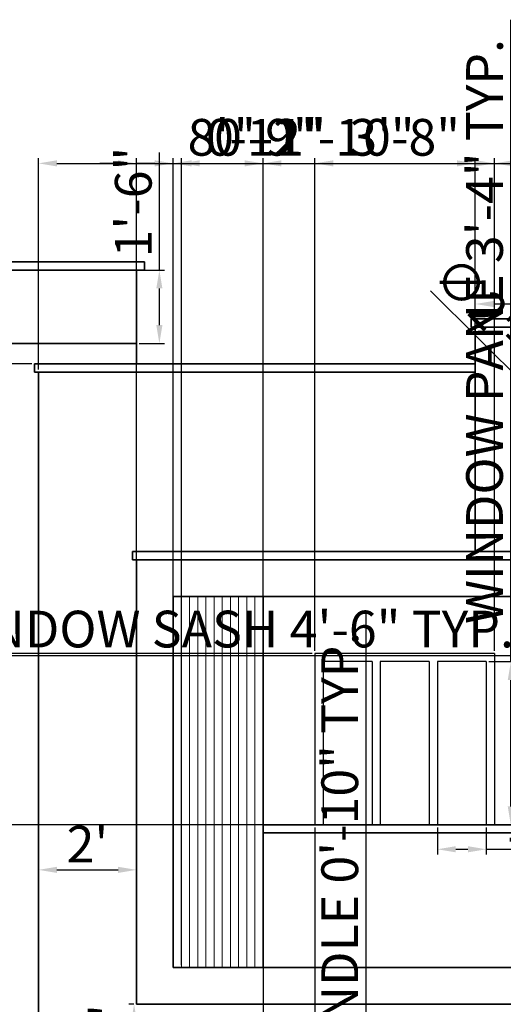
# Model space of a CAD drawing. Units: inches. Extents: x 3297 to 3846, y 520 to 959.
# Tile 4 of 5: x 3483 to 3602, y 717 to 959. Entities that reach past the tile are written whole.
import ezdxf

# ---------------------------------------------------------------- set-up
doc = ezdxf.new("R2010")
doc.units = ezdxf.units.IN
for name, color, linetype, lineweight in [('A-ANNO-DIMS', 2, 'Continuous', 18), ('A-ELEV', 7, 'Continuous', 35), ('A-ELEV-PATT', 8, 'Continuous', 13), ('A-GLAZ', 3, 'Continuous', 25)]:
    doc.layers.add(name, color=color, linetype=linetype, lineweight=lineweight)
doc.styles.get("Standard").update_dxf_attribs({"font": 'arial.ttf'})
doc.dimstyles.new('ISO-25', dxfattribs={"dimtxt": 9, "dimasz": 4.5, "dimexe": 1.25, "dimexo": 0.625, "dimtad": 1, "dimdec": 0, "dimlunit": 3, "dimtxsty": 'Standard', "dimcen": 2.5, "dimadec": 0, "dimazin": 0, "dimtfac": 1, "dimtdec": 0, "dimtmove": 0, "dimatfit": 3, "dimfxl": 1, "dimarcsym": 0})

# ---------------------------------------------------------------- blocks, each defined once
blk = doc.blocks.new('*D4')
at = {"layer": 'A-ANNO-DIMS', "color": 0, "lineweight": -2, "transparency": 16777216}
for p, q in [((3517.67, 897.24), (3517.67, 926.07)), ((3512.69, 897.24), (3518.92, 897.24)), ((3517.67, 883.74), (3517.67, 892.74)), ((3512.69, 879.24), (3518.92, 879.24))]:
    blk.add_line(p, q, dxfattribs=at)
at = {"layer": 'A-ANNO-DIMS', "color": 0, "transparency": 16777216}
for points in [[(3516.92, 892.74), (3518.42, 892.74), (3517.67, 897.24)], [(3516.92, 883.74), (3518.42, 883.74), (3517.67, 879.24)]]:
    blk.add_solid(points, dxfattribs=at)
at = {"layer": 'Defpoints', "color": 0, "transparency": 16777216}
for p in [(3512.06, 897.24), (3517.67, 897.24), (3512.06, 879.24)]:
    blk.add_point(p, dxfattribs=at)
at = {"layer": 'A-ANNO-DIMS', "color": 0, "transparency": 16777216, "insert": (3512.45, 913.9), "char_height": 9, "attachment_point": 5, "rotation": 90}
blk.add_mtext('1\'-6"', dxfattribs=at)
blk = doc.blocks.new('*D16')
at = {"layer": 'A-ANNO-DIMS', "color": 0, "lineweight": -2, "transparency": 16777216}
for p, q in [((3595.06, 874.87), (3595.06, 890.17)), ((3599.56, 888.92), (3650.56, 888.92)), ((3655.06, 874.87), (3655.06, 890.17))]:
    blk.add_line(p, q, dxfattribs=at)
at = {"layer": 'A-ANNO-DIMS', "color": 0, "transparency": 16777216}
for points in [[(3599.56, 889.67), (3599.56, 888.17), (3595.06, 888.92)], [(3650.56, 889.67), (3650.56, 888.17), (3655.06, 888.92)]]:
    blk.add_solid(points, dxfattribs=at)
at = {"layer": 'Defpoints', "color": 0, "transparency": 16777216}
for p in [(3655.06, 888.92), (3595.06, 874.24), (3655.06, 874.24)]:
    blk.add_point(p, dxfattribs=at)
at = {"layer": 'A-ANNO-DIMS', "color": 0, "transparency": 16777216, "insert": (3625.06, 894.12), "char_height": 9, "attachment_point": 5}
blk.add_mtext("5'", dxfattribs=at)
blk = doc.blocks.new('*D18')
at = {"layer": 'A-ANNO-DIMS', "color": 0, "lineweight": -2, "transparency": 16777216}
for p, q in [((3488.06, 746.43), (3488.06, 751.45)), ((3512.06, 746.43), (3512.06, 751.45)), ((3492.56, 750.2), (3507.56, 750.2))]:
    blk.add_line(p, q, dxfattribs=at)
at = {"layer": 'A-ANNO-DIMS', "color": 0, "transparency": 16777216}
for points in [[(3492.56, 750.95), (3492.56, 749.45), (3488.06, 750.2)], [(3507.56, 750.95), (3507.56, 749.45), (3512.06, 750.2)]]:
    blk.add_solid(points, dxfattribs=at)
at = {"layer": 'Defpoints', "color": 0, "transparency": 16777216}
for p in [(3512.06, 750.2), (3488.06, 745.81), (3512.06, 745.81)]:
    blk.add_point(p, dxfattribs=at)
at = {"layer": 'A-ANNO-DIMS', "color": 0, "transparency": 16777216, "insert": (3500.06, 755.34), "char_height": 9, "attachment_point": 5}
blk.add_mtext("2'", dxfattribs=at)
blk = doc.blocks.new('*D19')
at = {"layer": 'A-ANNO-DIMS', "color": 0, "lineweight": -2, "transparency": 16777216}
for p, q in [((3511.44, 717.24), (3510.23, 717.24)), ((3511.48, 712.74), (3511.48, 694.74)), ((3511.44, 690.24), (3510.23, 690.24))]:
    blk.add_line(p, q, dxfattribs=at)
at = {"layer": 'A-ANNO-DIMS', "color": 0, "transparency": 16777216}
for points in [[(3510.73, 712.74), (3512.23, 712.74), (3511.48, 717.24)], [(3510.73, 694.74), (3512.23, 694.74), (3511.48, 690.24)]]:
    blk.add_solid(points, dxfattribs=at)
at = {"layer": 'Defpoints', "color": 0, "transparency": 16777216}
for p in [(3512.06, 717.24), (3511.48, 690.24), (3512.06, 690.24)]:
    blk.add_point(p, dxfattribs=at)
at = {"layer": 'A-ANNO-DIMS', "color": 0, "transparency": 16777216, "insert": (3506.25, 703.74), "char_height": 9, "attachment_point": 5, "rotation": 90}
blk.add_mtext('2\'-3"', dxfattribs=at)
blk = doc.blocks.new('WIN-PANE')
for p, q in [((12, 40), (0, 40)), ((0, 40), (0, 0)), ((12, 40), (12, 0))]:
    blk.add_line(p, q)
blk = doc.blocks.new('*D27')
at = {"layer": 'A-ANNO-DIMS', "color": 0, "lineweight": -2, "transparency": 16777216}
for p, q in [((3603.76, 801.24), (3603.76, 958.61)), ((3598.39, 801.24), (3605.01, 801.24)), ((3603.76, 765.74), (3603.76, 796.74)), ((3598.39, 761.24), (3605.01, 761.24))]:
    blk.add_line(p, q, dxfattribs=at)
at = {"layer": 'A-ANNO-DIMS', "color": 0, "transparency": 16777216}
for points in [[(3603.01, 796.74), (3604.51, 796.74), (3603.76, 801.24)], [(3603.01, 765.74), (3604.51, 765.74), (3603.76, 761.24)]]:
    blk.add_solid(points, dxfattribs=at)
at = {"layer": 'Defpoints', "color": 0, "transparency": 16777216}
for p in [(3597.76, 801.24), (3603.76, 801.24), (3597.76, 761.24)]:
    blk.add_point(p, dxfattribs=at)
at = {"layer": 'A-ANNO-DIMS', "color": 0, "transparency": 16777216, "insert": (3598.48, 882.18), "char_height": 9, "attachment_point": 5, "rotation": 90}
blk.add_mtext('WINDOW PANE 3\'-4" TYP.', dxfattribs=at)
blk = doc.blocks.new('*D28')
at = {"layer": 'A-ANNO-DIMS', "color": 0, "lineweight": -2, "transparency": 16777216}
for p, q in [((3585.76, 760.62), (3585.76, 753.99)), ((3597.76, 760.62), (3597.76, 753.99)), ((3590.26, 755.24), (3593.26, 755.24)), ((3597.76, 755.24), (3657.53, 755.24))]:
    blk.add_line(p, q, dxfattribs=at)
at = {"layer": 'A-ANNO-DIMS', "color": 0, "transparency": 16777216}
for points in [[(3590.26, 755.99), (3590.26, 754.49), (3585.76, 755.24)], [(3593.26, 755.99), (3593.26, 754.49), (3597.76, 755.24)]]:
    blk.add_solid(points, dxfattribs=at)
at = {"layer": 'Defpoints', "color": 0, "transparency": 16777216}
for p in [(3585.76, 761.24), (3597.76, 761.24), (3597.76, 755.24)]:
    blk.add_point(p, dxfattribs=at)
at = {"layer": 'A-ANNO-DIMS', "color": 0, "transparency": 16777216, "insert": (3629.89, 760.46), "char_height": 9, "attachment_point": 5}
blk.add_mtext('1\'-0" TYP.', dxfattribs=at)
blk = doc.blocks.new('*D29')
at = {"layer": 'A-ANNO-DIMS', "color": 0, "lineweight": -2, "transparency": 16777216}
for p, q in [((3568.3, 650.24), (3568.3, 813.1)), ((3569.18, 645.74), (3567.05, 645.74)), ((3568.3, 635.74), (3568.3, 645.74)), ((3569.18, 635.74), (3567.05, 635.74)), ((3568.3, 631.24), (3568.3, 626.74))]:
    blk.add_line(p, q, dxfattribs=at)
at = {"layer": 'A-ANNO-DIMS', "color": 0, "transparency": 16777216}
for points in [[(3567.55, 650.24), (3569.05, 650.24), (3568.3, 645.74)], [(3567.55, 631.24), (3569.05, 631.24), (3568.3, 635.74)]]:
    blk.add_solid(points, dxfattribs=at)
at = {"layer": 'Defpoints', "color": 0, "transparency": 16777216}
for p in [(3568.3, 645.74), (3569.8, 645.74), (3569.8, 635.74)]:
    blk.add_point(p, dxfattribs=at)
at = {"layer": 'A-ANNO-DIMS', "color": 0, "transparency": 16777216, "insert": (3563.02, 733.92), "char_height": 9, "attachment_point": 5, "rotation": 90}
blk.add_mtext('DOOR HANDLE 0\'-10" TYP.', dxfattribs=at)
blk = doc.blocks.new('*D33')
at = {"layer": 'A-ANNO-DIMS', "color": 0, "lineweight": -2, "transparency": 16777216}
for p, q in [((3398.06, 795.31), (3398.06, 804.03)), ((3452.06, 795.31), (3452.06, 804.03)), ((3402.56, 802.78), (3447.56, 802.78)), ((3452.06, 802.78), (3609.43, 802.78))]:
    blk.add_line(p, q, dxfattribs=at)
at = {"layer": 'A-ANNO-DIMS', "color": 0, "transparency": 16777216}
for points in [[(3402.56, 803.53), (3402.56, 802.03), (3398.06, 802.78)], [(3447.56, 803.53), (3447.56, 802.03), (3452.06, 802.78)]]:
    blk.add_solid(points, dxfattribs=at)
at = {"layer": 'Defpoints', "color": 0, "transparency": 16777216}
for p in [(3452.06, 802.78), (3398.06, 794.68), (3452.06, 794.68)]:
    blk.add_point(p, dxfattribs=at)
at = {"layer": 'A-ANNO-DIMS', "color": 0, "transparency": 16777216, "insert": (3533, 808.06), "char_height": 9, "attachment_point": 5}
blk.add_mtext('WINDOW SASH 4\'-6" TYP.', dxfattribs=at)
blk = doc.blocks.new('*D43')
at = {"layer": 'A-ANNO-DIMS', "color": 0, "lineweight": -2, "transparency": 16777216}
for p, q in [((3488.06, 872.87), (3488.06, 924.64)), ((3595.06, 883.87), (3595.06, 924.64)), ((3492.56, 923.39), (3590.56, 923.39))]:
    blk.add_line(p, q, dxfattribs=at)
at = {"layer": 'A-ANNO-DIMS', "color": 0, "transparency": 16777216}
for points in [[(3492.56, 924.14), (3492.56, 922.64), (3488.06, 923.39)], [(3590.56, 924.14), (3590.56, 922.64), (3595.06, 923.39)]]:
    blk.add_solid(points, dxfattribs=at)
at = {"layer": 'Defpoints', "color": 0, "transparency": 16777216}
for p in [(3595.06, 923.39), (3595.06, 883.24), (3488.06, 872.24)]:
    blk.add_point(p, dxfattribs=at)
at = {"layer": 'A-ANNO-DIMS', "color": 0, "transparency": 16777216, "insert": (3541.56, 928.61), "char_height": 9, "attachment_point": 5}
blk.add_mtext('8\'-11"', dxfattribs=at)
blk = doc.blocks.new('*D64')
at = {"layer": 'A-ANNO-DIMS', "color": 0, "lineweight": -2, "transparency": 16777216}
for p, q in [((3512.06, 732.87), (3512.06, 924.64)), ((3521.06, 726.87), (3521.06, 924.64)), ((3507.56, 923.39), (3503.06, 923.39)), ((3512.06, 923.39), (3521.06, 923.39)), ((3525.56, 923.39), (3555.24, 923.39))]:
    blk.add_line(p, q, dxfattribs=at)
at = {"layer": 'A-ANNO-DIMS', "color": 0, "transparency": 16777216}
for points in [[(3507.56, 924.14), (3507.56, 922.64), (3512.06, 923.39)], [(3525.56, 924.14), (3525.56, 922.64), (3521.06, 923.39)]]:
    blk.add_solid(points, dxfattribs=at)
at = {"layer": 'Defpoints', "color": 0, "transparency": 16777216}
for p in [(3521.06, 923.39), (3512.06, 732.24), (3521.06, 726.24)]:
    blk.add_point(p, dxfattribs=at)
at = {"layer": 'A-ANNO-DIMS', "color": 0, "transparency": 16777216, "insert": (3542.65, 928.61), "char_height": 9, "attachment_point": 5}
blk.add_mtext('0\'-9"', dxfattribs=at)
blk = doc.blocks.new('*D65')
at = {"layer": 'A-ANNO-DIMS', "color": 0, "lineweight": -2, "transparency": 16777216}
for p, q in [((3521.06, 817.87), (3521.06, 924.64)), ((3543.06, 817.87), (3543.06, 924.64)), ((3525.56, 923.39), (3538.56, 923.39)), ((3543.06, 923.39), (3578.88, 923.39))]:
    blk.add_line(p, q, dxfattribs=at)
at = {"layer": 'A-ANNO-DIMS', "color": 0, "transparency": 16777216}
for points in [[(3525.56, 924.14), (3525.56, 922.64), (3521.06, 923.39)], [(3538.56, 924.14), (3538.56, 922.64), (3543.06, 923.39)]]:
    blk.add_solid(points, dxfattribs=at)
at = {"layer": 'Defpoints', "color": 0, "transparency": 16777216}
for p in [(3543.06, 923.39), (3521.06, 817.24), (3543.06, 817.24)]:
    blk.add_point(p, dxfattribs=at)
at = {"layer": 'A-ANNO-DIMS', "color": 0, "transparency": 16777216, "insert": (3563.22, 928.61), "char_height": 9, "attachment_point": 5}
blk.add_mtext('1\'-10"', dxfattribs=at)
blk = doc.blocks.new('*D66')
at = {"layer": 'A-ANNO-DIMS', "color": 0, "lineweight": -2, "transparency": 16777216}
for p, q in [((3521.06, 726.87), (3521.06, 924.64)), ((3523.06, 726.87), (3523.06, 924.64)), ((3516.56, 923.39), (3512.06, 923.39)), ((3521.06, 923.39), (3523.06, 923.39)), ((3527.56, 923.39), (3557.24, 923.39))]:
    blk.add_line(p, q, dxfattribs=at)
at = {"layer": 'A-ANNO-DIMS', "color": 0, "transparency": 16777216}
for points in [[(3516.56, 924.14), (3516.56, 922.64), (3521.06, 923.39)], [(3527.56, 924.14), (3527.56, 922.64), (3523.06, 923.39)]]:
    blk.add_solid(points, dxfattribs=at)
at = {"layer": 'Defpoints', "color": 0, "transparency": 16777216}
for p in [(3523.06, 923.39), (3521.06, 726.24), (3523.06, 726.24)]:
    blk.add_point(p, dxfattribs=at)
at = {"layer": 'A-ANNO-DIMS', "color": 0, "transparency": 16777216, "insert": (3544.65, 928.61), "char_height": 9, "attachment_point": 5}
blk.add_mtext('0\'-2"', dxfattribs=at)
blk = doc.blocks.new('*D69')
at = {"layer": 'A-ANNO-DIMS', "color": 0, "lineweight": -2, "transparency": 16777216}
for p, q in [((3543.06, 759.87), (3543.06, 924.64)), ((3748.06, 761.87), (3748.06, 924.64)), ((3547.56, 923.39), (3743.56, 923.39))]:
    blk.add_line(p, q, dxfattribs=at)
at = {"layer": 'A-ANNO-DIMS', "color": 0, "transparency": 16777216}
for points in [[(3547.56, 924.14), (3547.56, 922.64), (3543.06, 923.39)], [(3743.56, 924.14), (3743.56, 922.64), (3748.06, 923.39)]]:
    blk.add_solid(points, dxfattribs=at)
at = {"layer": 'Defpoints', "color": 0, "transparency": 16777216}
for p in [(3748.06, 923.39), (3748.06, 761.24), (3543.06, 759.24)]:
    blk.add_point(p, dxfattribs=at)
at = {"layer": 'A-ANNO-DIMS', "color": 0, "transparency": 16777216, "insert": (3645.56, 928.53), "char_height": 9, "attachment_point": 5}
blk.add_mtext('17\'-1"', dxfattribs=at)
blk = doc.blocks.new('*D70')
at = {"layer": 'A-ANNO-DIMS', "color": 0, "lineweight": -2, "transparency": 16777216}
for p, q in [((3555.76, 760.62), (3555.76, 526.84)), ((3543.06, 758.62), (3543.06, 526.84)), ((3547.56, 528.09), (3551.26, 528.09)), ((3555.76, 528.09), (3605.56, 528.09))]:
    blk.add_line(p, q, dxfattribs=at)
at = {"layer": 'A-ANNO-DIMS', "color": 0, "transparency": 16777216}
for points in [[(3547.56, 528.84), (3547.56, 527.34), (3543.06, 528.09)], [(3551.26, 528.84), (3551.26, 527.34), (3555.76, 528.09)]]:
    blk.add_solid(points, dxfattribs=at)
at = {"layer": 'Defpoints', "color": 0, "transparency": 16777216}
for p in [(3555.76, 761.24), (3543.06, 759.24), (3555.76, 528.09)]:
    blk.add_point(p, dxfattribs=at)
at = {"layer": 'A-ANNO-DIMS', "color": 0, "transparency": 16777216, "insert": (3582.91, 533.37), "char_height": 9, "attachment_point": 5}
blk.add_mtext('1\'-0 1/2"', dxfattribs=at)
blk = doc.blocks.new('*D71')
at = {"layer": 'A-ANNO-DIMS', "color": 0, "lineweight": -2, "transparency": 16777216}
for p, q in [((3555.76, 803.87), (3555.76, 924.64)), ((3599.76, 803.87), (3599.76, 924.64)), ((3560.26, 923.39), (3595.26, 923.39))]:
    blk.add_line(p, q, dxfattribs=at)
at = {"layer": 'A-ANNO-DIMS', "color": 0, "transparency": 16777216}
for points in [[(3560.26, 924.14), (3560.26, 922.64), (3555.76, 923.39)], [(3595.26, 924.14), (3595.26, 922.64), (3599.76, 923.39)]]:
    blk.add_solid(points, dxfattribs=at)
at = {"layer": 'Defpoints', "color": 0, "transparency": 16777216}
for p in [(3599.76, 923.39), (3555.76, 803.24), (3599.76, 803.24)]:
    blk.add_point(p, dxfattribs=at)
at = {"layer": 'A-ANNO-DIMS', "color": 0, "transparency": 16777216, "insert": (3577.76, 928.61), "char_height": 9, "attachment_point": 5}
blk.add_mtext('3\'-8"', dxfattribs=at)
blk = doc.blocks.new('*D72')
at = {"layer": 'A-ANNO-DIMS', "color": 0, "lineweight": -2, "transparency": 16777216}
for p, q in [((3555.14, 803.24), (3306.66, 803.24)), ((3307.91, 765.74), (3307.91, 798.74)), ((3555.14, 761.24), (3306.66, 761.24))]:
    blk.add_line(p, q, dxfattribs=at)
at = {"layer": 'A-ANNO-DIMS', "color": 0, "transparency": 16777216}
for points in [[(3307.16, 798.74), (3308.66, 798.74), (3307.91, 803.24)], [(3307.16, 765.74), (3308.66, 765.74), (3307.91, 761.24)]]:
    blk.add_solid(points, dxfattribs=at)
at = {"layer": 'Defpoints', "color": 0, "transparency": 16777216}
for p in [(3307.91, 803.24), (3555.76, 803.24), (3555.76, 761.24)]:
    blk.add_point(p, dxfattribs=at)
at = {"layer": 'A-ANNO-DIMS', "color": 0, "transparency": 16777216, "insert": (3302.69, 782.24), "char_height": 9, "attachment_point": 5, "rotation": 90}
blk.add_mtext('3\'-6"', dxfattribs=at)
blk = doc.blocks.new('*D73')
at = {"layer": 'A-ANNO-DIMS', "color": 0, "lineweight": -2, "transparency": 16777216}
for p, q in [((3599.76, 803.87), (3599.76, 924.64)), ((3678.06, 803.87), (3678.06, 924.64)), ((3604.26, 923.39), (3673.56, 923.39))]:
    blk.add_line(p, q, dxfattribs=at)
at = {"layer": 'A-ANNO-DIMS', "color": 0, "transparency": 16777216}
for points in [[(3604.26, 924.14), (3604.26, 922.64), (3599.76, 923.39)], [(3673.56, 924.14), (3673.56, 922.64), (3678.06, 923.39)]]:
    blk.add_solid(points, dxfattribs=at)
at = {"layer": 'Defpoints', "color": 0, "transparency": 16777216}
for p in [(3678.06, 923.39), (3599.76, 803.24), (3678.06, 803.24)]:
    blk.add_point(p, dxfattribs=at)
at = {"layer": 'A-ANNO-DIMS', "color": 0, "transparency": 16777216, "insert": (3638.91, 928.67), "char_height": 9, "attachment_point": 5}
blk.add_mtext('6\'-6 1/2"', dxfattribs=at)
blk = doc.blocks.new('*D78')
at = {"layer": 'A-ANNO-DIMS', "color": 0, "lineweight": -2, "transparency": 16777216}
for p, q in [((3307.91, 899.24), (3307.91, 929.07)), ((3513.44, 899.24), (3306.66, 899.24)), ((3307.91, 878.74), (3307.91, 894.74)), ((3486.44, 874.24), (3306.66, 874.24))]:
    blk.add_line(p, q, dxfattribs=at)
at = {"layer": 'A-ANNO-DIMS', "color": 0, "transparency": 16777216}
for points in [[(3307.16, 894.74), (3308.66, 894.74), (3307.91, 899.24)], [(3307.16, 878.74), (3308.66, 878.74), (3307.91, 874.24)]]:
    blk.add_solid(points, dxfattribs=at)
at = {"layer": 'Defpoints', "color": 0, "transparency": 16777216}
for p in [(3307.91, 899.24), (3514.06, 899.24), (3487.06, 874.24)]:
    blk.add_point(p, dxfattribs=at)
at = {"layer": 'A-ANNO-DIMS', "color": 0, "transparency": 16777216, "insert": (3302.77, 916.41), "char_height": 9, "attachment_point": 5, "rotation": 90}
blk.add_mtext('2\'-1"', dxfattribs=at)
blk = doc.blocks.new('*D82')
at = {"layer": 'A-ANNO-DIMS', "color": 0, "lineweight": -2, "transparency": 16777216}
for p, q in [((3584.1, 892.18), (3612.02, 864.28)), ((3634.93, 841.38), (3615.2, 861.1)), ((3638.11, 838.2), (3641.3, 835.02))]:
    blk.add_line(p, q, dxfattribs=at)
at = {"layer": 'A-ANNO-DIMS', "color": 0, "transparency": 16777216}
for points in [[(3612.55, 864.81), (3611.49, 863.75), (3615.2, 861.1)], [(3638.64, 838.73), (3637.58, 837.67), (3634.93, 841.38)]]:
    blk.add_solid(points, dxfattribs=at)
at = {"layer": 'Defpoints', "color": 0, "transparency": 16777216}
for p in [(3615.2, 861.1), (3634.93, 841.38)]:
    blk.add_point(p, dxfattribs=at)
at = {"layer": 'A-ANNO-DIMS', "color": 0, "transparency": 16777216, "insert": (3600.34, 883.69), "char_height": 9, "attachment_point": 5, "rotation": 315.0171}
blk.add_mtext('∅2\'-4"', dxfattribs=at)

msp = doc.modelspace()

# ---------------------------------------------------------------- linework, layer by layer
at = {"layer": 'A-ELEV'}
for p, q in [((3332.06, 899.24), (3514.06, 899.24)), ((3514.06, 897.24), (3514.06, 899.24)), ((3332.06, 897.24), (3514.06, 897.24)), ((3512.06, 874.24), (3512.06, 897.24)), ((3594.06, 885.24), (3656.06, 885.24)), ((3594.06, 885.24), (3594.06, 883.24)), ((3594.06, 883.24), (3656.06, 883.24)), ((3595.06, 883.24), (3595.06, 828.24)), ((3350.06, 879.24), (3512.06, 879.24)), ((3487.06, 874.24), (3595.06, 874.24)), ((3487.06, 872.24), (3487.06, 874.24)), ((3487.06, 872.24), (3595.06, 872.24)), ((3488.06, 690.24), (3488.06, 872.24)), ((3512.06, 828.24), (3511.12, 828.24)), ((3511.12, 826.24), (3511.12, 828.24)), ((3512.06, 828.24), (3753.06, 828.24)), ((3512.06, 826.24), (3511.12, 826.24)), ((3512.06, 732.24), (3512.06, 826.24)), ((3512.06, 826.24), (3753.06, 826.24)), ((3512.06, 826.24), (3512.06, 717.24)), ((3521.06, 817.24), (3752.06, 817.24)), ((3521.06, 726.24), (3521.06, 817.24)), ((3543.06, 726.24), (3543.06, 817.24)), ((3543.06, 761.24), (3748.06, 761.24)), ((3543.06, 759.24), (3746.06, 759.24)), ((3521.06, 726.24), (3752.06, 726.24)), ((3512.06, 717.24), (3752.06, 717.24))]:
    msp.add_line(p, q, dxfattribs=at)
at = {"layer": 'A-ELEV-PATT'}
for p, q in [((3523.06, 726.24), (3523.06, 817.24)), ((3525.06, 726.24), (3525.06, 817.24)), ((3527.06, 726.24), (3527.06, 817.24)), ((3529.06, 726.24), (3529.06, 817.24)), ((3531.06, 726.24), (3531.06, 817.24)), ((3533.06, 726.24), (3533.06, 817.24)), ((3535.06, 726.24), (3535.06, 817.24)), ((3537.06, 726.24), (3537.06, 817.24)), ((3539.06, 726.24), (3539.06, 817.24)), ((3541.06, 726.24), (3541.06, 817.24))]:
    msp.add_line(p, q, dxfattribs=at)
at = {"layer": 'A-GLAZ'}
for p, q in [((3599.76, 803.24), (3555.76, 803.24)), ((3555.76, 803.24), (3555.76, 761.24)), ((3599.76, 803.24), (3599.76, 761.24))]:
    msp.add_line(p, q, dxfattribs=at)

# ---------------------------------------------------------------- block references
for p in [(3557.76, 761.24), (3571.76, 761.24), (3585.76, 761.24)]:
    msp.add_blockref('WIN-PANE', p, dxfattribs=at)

# ---------------------------------------------------------------- dimensions: what is measured, and where the dimension line sits
at = {"layer": 'A-ANNO-DIMS'}
for base, p1, p2, text, picture, middle in [((3603.76, 801.24), (3597.76, 761.24), (3597.76, 801.24), 'WINDOW PANE <> TYP.', '*D27', (3598.48, 882.18)), ((3568.3, 645.74), (3569.8, 635.74), (3569.8, 645.74), 'DOOR HANDLE <> TYP.', '*D29', (3563.02, 733.92))]:
    dim = msp.add_linear_dim(base=base, p1=p1, p2=p2, angle=90, text=text, dimstyle='ISO-25', override={"dimdec": 1, "dimrnd": 0, "dimzin": 1, "dimlunit": 4, "dimfrac": 2}, dxfattribs=at)
    dim.commit()
    dim.dimension.update_dxf_attribs({"geometry": picture, "text_midpoint": middle})
for base, p1, p2, override, picture, middle in [((3678.06, 923.39), (3599.76, 803.24), (3678.06, 803.24), {"dimdec": 1, "dimlfac": 1, "dimrnd": 0, "dimzin": 1, "dimdsep": 46, "dimlunit": 4, "dimfrac": 2}, '*D73', (3638.91, 928.67)), ((3595.06, 923.39), (3488.06, 872.24), (3595.06, 883.24), {"dimdec": 1, "dimlfac": 1, "dimrnd": 0, "dimzin": 1, "dimdsep": 46, "dimlunit": 4, "dimfrac": 2}, '*D43', (3541.56, 928.61)), ((3521.06, 923.39), (3512.06, 732.24), (3521.06, 726.24), {"dimdec": 1, "dimlfac": 1, "dimrnd": 0, "dimzin": 1, "dimdsep": 46, "dimlunit": 4, "dimfrac": 2}, '*D64', (3542.65, 928.61)), ((3523.06, 923.39), (3521.06, 726.24), (3523.06, 726.24), {"dimdec": 1, "dimlfac": 1, "dimrnd": 0, "dimzin": 1, "dimdsep": 46, "dimlunit": 4, "dimfrac": 2}, '*D66', (3544.65, 928.61)), ((3543.06, 923.39), (3521.06, 817.24), (3543.06, 817.24), {"dimdec": 1, "dimlfac": 1, "dimrnd": 0, "dimzin": 1, "dimdsep": 46, "dimlunit": 4, "dimfrac": 2}, '*D65', (3563.22, 928.61)), ((3748.06, 923.39), (3543.06, 759.24), (3748.06, 761.24), {"dimdec": 1, "dimlfac": 1, "dimrnd": 0, "dimzin": 1, "dimdsep": 46, "dimlunit": 4, "dimfrac": 2}, '*D69', (3645.56, 928.53)), ((3599.76, 923.39), (3555.76, 803.24), (3599.76, 803.24), {"dimdec": 1, "dimlfac": 1, "dimrnd": 0, "dimzin": 1, "dimdsep": 46, "dimlunit": 4, "dimfrac": 2}, '*D71', (3577.76, 928.61)), ((3655.06, 888.92), (3595.06, 874.24), (3655.06, 874.24), {"dimclrd": 0, "dimclre": 0, "dimclrt": 0}, '*D16', (3625.06, 894.12)), ((3512.06, 750.2), (3488.06, 745.81), (3512.06, 745.81), {"dimclrd": 0, "dimclre": 0, "dimclrt": 0}, '*D18', (3500.06, 755.34)), ((3555.76, 528.09), (3543.06, 759.24), (3555.76, 761.24), {"dimdec": 1, "dimlfac": 1, "dimrnd": 0, "dimzin": 1, "dimdsep": 46, "dimlunit": 4, "dimfrac": 2}, '*D70', (3582.91, 533.37))]:
    dim = msp.add_linear_dim(base=base, p1=p1, p2=p2, dimstyle='ISO-25', override=override, dxfattribs=at)
    dim.commit()
    dim.dimension.update_dxf_attribs({"geometry": picture, "text_midpoint": middle})
for base, p1, p2, override, picture, middle in [((3307.91, 899.24), (3487.06, 874.24), (3514.06, 899.24), {"dimdec": 1, "dimlfac": 1, "dimrnd": 0, "dimzin": 1, "dimdsep": 46, "dimlunit": 4, "dimfrac": 2}, '*D78', (3302.77, 916.41)), ((3517.67, 897.24), (3512.06, 879.24), (3512.06, 897.24), {"dimclrd": 0, "dimclre": 0, "dimclrt": 0}, '*D4', (3512.45, 913.9)), ((3307.91, 803.24), (3555.76, 761.24), (3555.76, 803.24), {"dimdec": 1, "dimlfac": 1, "dimrnd": 0, "dimzin": 1, "dimdsep": 46, "dimlunit": 4, "dimfrac": 2}, '*D72', (3302.69, 782.24)), ((3511.48, 690.24), (3512.06, 717.24), (3512.06, 690.24), {"dimclrd": 0, "dimclre": 0, "dimclrt": 0}, '*D19', (3506.25, 703.74))]:
    dim = msp.add_linear_dim(base=base, p1=p1, p2=p2, angle=90, dimstyle='ISO-25', override=override, dxfattribs=at)
    dim.commit()
    dim.dimension.update_dxf_attribs({"geometry": picture, "text_midpoint": middle})
dim = msp.add_diameter_dim_2p(p1=(3634.93, 841.38), p2=(3615.2, 861.1), dimstyle='ISO-25', override={"dimdec": 1, "dimlfac": 1, "dimrnd": 0, "dimzin": 1, "dimdsep": 46, "dimlunit": 4, "dimfrac": 2}, dxfattribs=at)
dim.commit()
dim.dimension.update_dxf_attribs({"geometry": '*D82', "text_midpoint": (3596.47, 879.82), "dimtype": 163})
for base, p1, p2, text, picture, middle in [((3452.06, 802.78), (3398.06, 794.68), (3452.06, 794.68), 'WINDOW SASH <> TYP.', '*D33', (3533, 808.06)), ((3597.76, 755.24), (3585.76, 761.24), (3597.76, 761.24), '<> TYP.', '*D28', (3629.89, 760.46))]:
    dim = msp.add_linear_dim(base=base, p1=p1, p2=p2, text=text, dimstyle='ISO-25', override={"dimdec": 1, "dimrnd": 0, "dimzin": 1, "dimlunit": 4, "dimfrac": 2}, dxfattribs=at)
    dim.commit()
    dim.dimension.update_dxf_attribs({"geometry": picture, "text_midpoint": middle})

doc.saveas('drawing.dxf')
